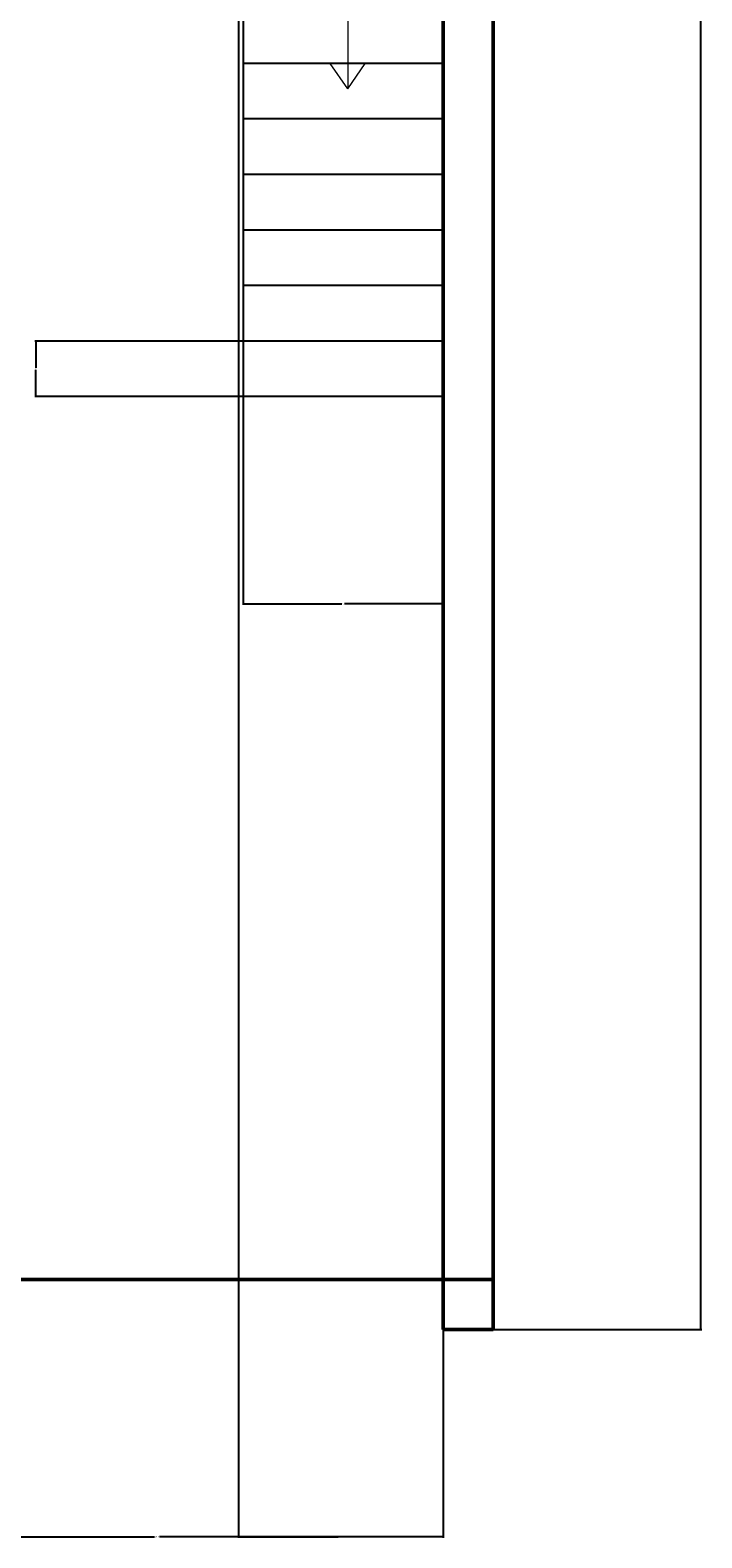
# Model space of a CAD drawing. Units: inches. Extents: x 383 to 970, y 275 to 1088.
# Tile 4 of 11: x 849 to 970, y 275 to 546. Entities that reach past the tile are written whole.
import ezdxf

# ---------------------------------------------------------------- set-up
doc = ezdxf.new("R2010")
doc.units = ezdxf.units.IN
doc.header["$MEASUREMENT"] = 0
for name, color, linetype, lineweight in [('A-ANNO-DIMS', 2, 'Continuous', 18), ('A-ANNO-SYMB', 7, 'Continuous', 18), ('A-FLOR-STRS', 7, 'Continuous', 25), ('A-WALL', 7, 'Continuous', 50)]:
    doc.layers.add(name, color=color, linetype=linetype, lineweight=lineweight)
doc.styles.get("Standard").update_dxf_attribs({"font": 'arial.ttf'})
doc.dimstyles.get("Standard").update_dxf_attribs({"dimtxt": 0.18, "dimasz": 0.18, "dimexe": 0.18, "dimexo": 0.0625, "dimgap": 0.09, "dimtad": 0, "dimtih": 1, "dimtoh": 1, "dimdec": 4, "dimzin": 0, "dimdsep": 46, "dimtxsty": 'Standard', "dimcen": 0.09, "dimadec": 0, "dimazin": 0, "dimtfac": 1, "dimtdec": 4, "dimtofl": 0, "dimtmove": 0, "dimatfit": 3, "dimfxl": 1, "dimtolj": 1, "dimtzin": 0, "dimarcsym": 0})

# ---------------------------------------------------------------- blocks, each defined once
blk = doc.blocks.new('*D38')
at = {"layer": 'A-ANNO-DIMS', "color": 0, "lineweight": -2, "transparency": 16777216}
for p, q in [((932.3, 1050.14), (969.77, 1050.14)), ((969.59, 1049.96), (969.59, 681.32)), ((969.59, 312.32), (969.59, 680.95)), ((932.3, 312.14), (969.77, 312.14))]:
    blk.add_line(p, q, dxfattribs=at)
at = {"layer": 'A-ANNO-DIMS', "color": 0, "transparency": 16777216}
for points in [[(969.56, 1049.96), (969.62, 1049.96), (969.59, 1050.14)], [(969.56, 312.32), (969.62, 312.32), (969.59, 312.14)]]:
    blk.add_solid(points, dxfattribs=at)
at = {"layer": 'Defpoints', "color": 0, "transparency": 16777216}
for p in [(932.24, 1050.14), (969.59, 1050.14), (932.24, 312.14)]:
    blk.add_point(p, dxfattribs=at)
at = {"layer": 'A-ANNO-DIMS', "color": 0, "transparency": 16777216, "insert": (969.59, 681.14), "char_height": 0.18, "attachment_point": 5}
blk.add_mtext('\\A1;738', dxfattribs=at)
blk = doc.blocks.new('*D45')
at = {"layer": 'A-ANNO-DIMS', "color": 0, "lineweight": -2, "transparency": 16777216}
for p, q in [((820.18, 312.07), (820.18, 274.61)), ((923.24, 312.07), (923.24, 274.61)), ((820.36, 274.79), (871.26, 274.79)), ((923.06, 274.79), (872.17, 274.79))]:
    blk.add_line(p, q, dxfattribs=at)
at = {"layer": 'A-ANNO-DIMS', "color": 0, "transparency": 16777216}
for points in [[(820.36, 274.82), (820.36, 274.76), (820.18, 274.79)], [(923.06, 274.82), (923.06, 274.76), (923.24, 274.79)]]:
    blk.add_solid(points, dxfattribs=at)
at = {"layer": 'Defpoints', "color": 0, "transparency": 16777216}
for p in [(820.18, 312.14), (923.24, 312.14), (923.24, 274.79)]:
    blk.add_point(p, dxfattribs=at)
at = {"layer": 'A-ANNO-DIMS', "color": 0, "transparency": 16777216, "insert": (871.71, 274.79), "char_height": 0.18, "attachment_point": 5}
blk.add_mtext('\\A1;103.06', dxfattribs=at)
blk = doc.blocks.new('*D46')
at = {"layer": 'A-ANNO-DIMS', "color": 0, "lineweight": -2, "transparency": 16777216}
for p, q in [((887.18, 490.14), (849.71, 490.14)), ((849.89, 489.96), (849.89, 485.32)), ((849.89, 480.32), (849.89, 484.95)), ((887.18, 480.14), (849.71, 480.14))]:
    blk.add_line(p, q, dxfattribs=at)
at = {"layer": 'A-ANNO-DIMS', "color": 0, "transparency": 16777216}
for points in [[(849.86, 489.96), (849.92, 489.96), (849.89, 490.14)], [(849.86, 480.32), (849.92, 480.32), (849.89, 480.14)]]:
    blk.add_solid(points, dxfattribs=at)
at = {"layer": 'Defpoints', "color": 0, "transparency": 16777216}
for p in [(849.89, 490.14), (887.24, 490.14), (887.24, 480.14)]:
    blk.add_point(p, dxfattribs=at)
at = {"layer": 'A-ANNO-DIMS', "color": 0, "transparency": 16777216, "insert": (849.89, 485.14), "char_height": 0.18, "attachment_point": 5}
blk.add_mtext('\\A1;10', dxfattribs=at)
blk = doc.blocks.new('*D47')
at = {"layer": 'A-ANNO-DIMS', "color": 0, "lineweight": -2, "transparency": 16777216}
for p, q in [((887.24, 480.07), (887.24, 442.61)), ((923.24, 480.07), (923.24, 442.61)), ((887.42, 442.79), (905.02, 442.79)), ((923.06, 442.79), (905.46, 442.79))]:
    blk.add_line(p, q, dxfattribs=at)
at = {"layer": 'A-ANNO-DIMS', "color": 0, "transparency": 16777216}
for points in [[(887.42, 442.82), (887.42, 442.76), (887.24, 442.79)], [(923.06, 442.82), (923.06, 442.76), (923.24, 442.79)]]:
    blk.add_solid(points, dxfattribs=at)
at = {"layer": 'Defpoints', "color": 0, "transparency": 16777216}
for p in [(887.24, 480.14), (923.24, 480.14), (887.24, 442.79)]:
    blk.add_point(p, dxfattribs=at)
at = {"layer": 'A-ANNO-DIMS', "color": 0, "transparency": 16777216, "insert": (905.24, 442.79), "char_height": 0.18, "attachment_point": 5}
blk.add_mtext('\\A1;36', dxfattribs=at)
blk = doc.blocks.new('*D55')
at = {"layer": 'A-ANNO-DIMS', "color": 0, "lineweight": -2, "transparency": 16777216}
for p, q in [((886.41, 644.89), (886.41, 274.61)), ((923.24, 615.07), (923.24, 274.61)), ((886.59, 274.79), (904.36, 274.79)), ((923.06, 274.79), (905.29, 274.79))]:
    blk.add_line(p, q, dxfattribs=at)
at = {"layer": 'A-ANNO-DIMS', "color": 0, "transparency": 16777216}
for points in [[(886.59, 274.82), (886.59, 274.76), (886.41, 274.79)], [(923.06, 274.82), (923.06, 274.76), (923.24, 274.79)]]:
    blk.add_solid(points, dxfattribs=at)
at = {"layer": 'Defpoints', "color": 0, "transparency": 16777216}
for p in [(886.41, 644.96), (923.24, 615.14), (923.24, 274.79)]:
    blk.add_point(p, dxfattribs=at)
at = {"layer": 'A-ANNO-DIMS', "color": 0, "transparency": 16777216, "insert": (904.82, 274.79), "char_height": 0.18, "attachment_point": 5}
blk.add_mtext('\\A1;36.834', dxfattribs=at)

msp = doc.modelspace()

# ---------------------------------------------------------------- linework, layer by layer
at = {"layer": 'A-ANNO-SYMB'}
for p, q in [((906.0568, 588.7988), (906.0568, 535.5591)), ((906.0568, 535.5591), (902.8927, 540.1365)), ((906.0568, 535.5591), (909.2208, 540.1365))]:
    msp.add_line(p, q, dxfattribs=at)
at = {"layer": 'A-FLOR-STRS'}
for p, q in [((887.24, 606.1365), (887.24, 475.2293)), ((923.24, 540.1365), (887.24, 540.1365)), ((923.24, 530.1365), (887.24, 530.1365)), ((923.24, 520.1365), (887.24, 520.1365)), ((923.24, 510.1365), (887.24, 510.1365)), ((923.24, 500.1365), (887.24, 500.1365)), ((923.24, 490.1365), (887.24, 490.1365)), ((923.24, 480.1365), (887.24, 480.1365))]:
    msp.add_line(p, q, dxfattribs=at)
at = {"layer": 'A-WALL'}
for p, q in [((932.24, 1050.1365), (932.24, 312.1365)), ((923.24, 606.1365), (923.24, 312.1365)), ((820.1849, 321.1365), (932.24, 321.1365)), ((923.24, 312.1365), (932.24, 312.1365))]:
    msp.add_line(p, q, dxfattribs=at)

# ---------------------------------------------------------------- dimensions: what is measured, and where the dimension line sits
at = {"layer": 'A-ANNO-DIMS'}
for base, p1, p2, angle, picture, middle in [((969.59, 1050.1365), (932.24, 312.1365), (932.24, 1050.1365), 90, '*D38', (969.59, 681.1365)), ((849.89, 490.1365), (887.24, 480.1365), (887.24, 490.1365), 90, '*D46', (849.89, 485.1365)), ((887.24, 442.7865), (923.24, 480.1365), (887.24, 480.1365), 180, '*D47', (905.24, 442.7865))]:
    dim = msp.add_linear_dim(base=base, p1=p1, p2=p2, angle=angle, dimstyle='Standard', override={"dimdec": 0, "dimlfac": 1, "dimrnd": 0, "dimzin": 0, "dimdsep": 46, "dimlunit": 2}, dxfattribs=at)
    dim.commit()
    dim.dimension.update_dxf_attribs({"geometry": picture, "text_midpoint": middle})
for p1, p2, override, picture, middle in [((886.4057, 644.9565), (923.24, 615.1365), {"dimdec": 3, "dimlfac": 1, "dimrnd": 0, "dimzin": 0, "dimdsep": 46, "dimlunit": 2}, '*D55', (904.8229, 274.7865)), ((820.1849, 312.1365), (923.24, 312.1365), {"dimdec": 2, "dimlfac": 1, "dimrnd": 0, "dimzin": 0, "dimdsep": 46, "dimlunit": 2}, '*D45', (871.7125, 274.7865))]:
    dim = msp.add_linear_dim(base=(923.24, 274.7865), p1=p1, p2=p2, dimstyle='Standard', override=override, dxfattribs=at)
    dim.commit()
    dim.dimension.update_dxf_attribs({"geometry": picture, "text_midpoint": middle})

doc.saveas('drawing.dxf')
